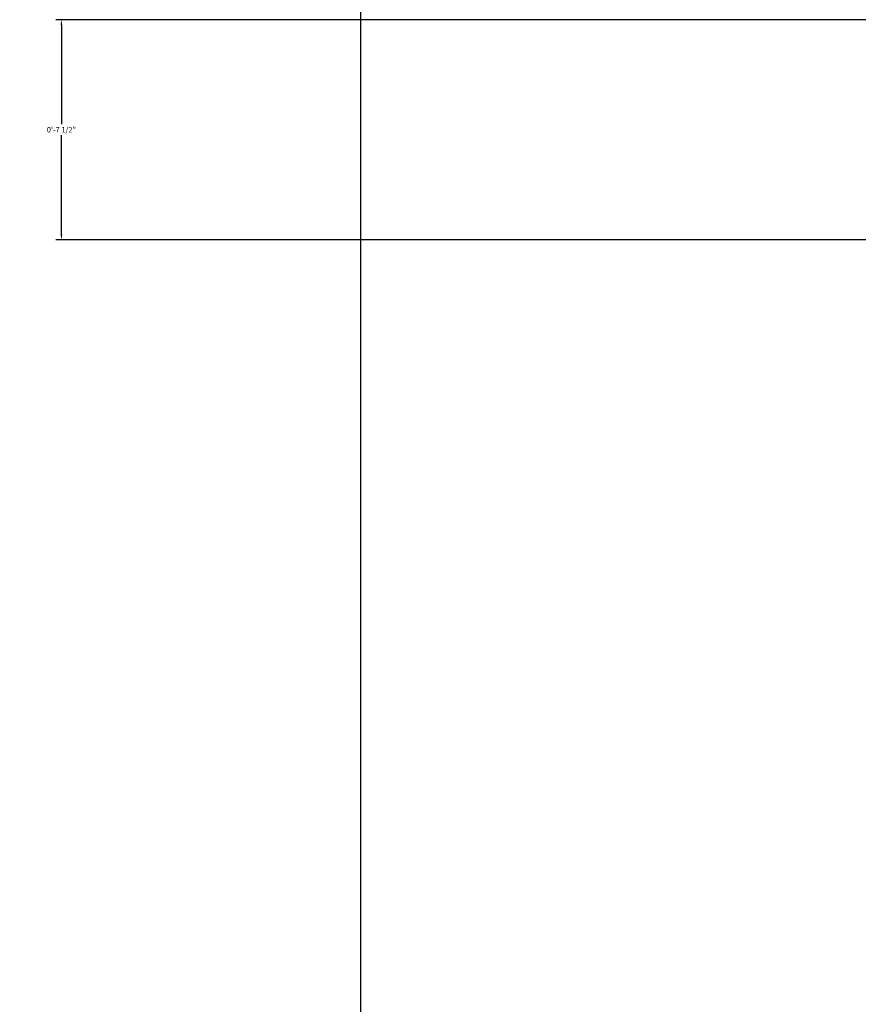
# Model space of a CAD drawing. Units: inches. Extents: x -5 to 330, y -522 to 40.
# Tile 9 of 23: x -5 to 23, y -330 to -297. Entities that reach past the tile are written whole.
import ezdxf

# ---------------------------------------------------------------- set-up
doc = ezdxf.new("R2010")
doc.units = ezdxf.units.IN
doc.header["$MEASUREMENT"] = 0
doc.layers.add('A-ANNO-DIMS', color=2, linetype='Continuous', lineweight=18)
doc.styles.get("Standard").update_dxf_attribs({"font": 'arial.ttf'})
doc.dimstyles.get("Standard").update_dxf_attribs({"dimtxt": 0.18, "dimasz": 0.18, "dimexe": 0.18, "dimexo": 0.0625, "dimgap": 0.09, "dimtad": 0, "dimtih": 1, "dimtoh": 1, "dimdec": 0, "dimzin": 0, "dimdsep": 46, "dimlunit": 3, "dimtxsty": 'Standard', "dimcen": 0.09, "dimadec": 0, "dimazin": 0, "dimtfac": 1, "dimtdec": 0, "dimtofl": 0, "dimtmove": 0, "dimatfit": 3, "dimfxl": 1, "dimtolj": 1, "dimtzin": 0, "dimarcsym": 0})

# ---------------------------------------------------------------- blocks, each defined once
blk = doc.blocks.new('*D2')
at = {"layer": 'A-ANNO-DIMS', "color": 0, "lineweight": -2, "transparency": 16777216}
for p, q in [((23.447, 12.356), (6.274, 12.356)), ((6.454, 12.176), (6.454, -203.738)), ((6.454, -425.964), (6.454, -210.049)), ((23.447, -426.144), (6.274, -426.144))]:
    blk.add_line(p, q, dxfattribs=at)
at = {"layer": 'A-ANNO-DIMS', "color": 0, "transparency": 16777216}
for points in [[(6.424, 12.176), (6.484, 12.176), (6.454, 12.356)], [(6.424, -425.964), (6.484, -425.964), (6.454, -426.144)]]:
    blk.add_solid(points, dxfattribs=at)
at = {"layer": 'Defpoints', "color": 0, "transparency": 16777216}
for p in [(23.51, 12.356), (6.454, -426.144), (23.51, -426.144)]:
    blk.add_point(p, dxfattribs=at)
at = {"layer": 'A-ANNO-DIMS', "color": 0, "transparency": 16777216, "insert": (6.454, -206.894), "char_height": 6, "attachment_point": 5}
blk.add_mtext('\\A1;36\'-7"', dxfattribs=at)
blk = doc.blocks.new('*D47')
at = {"layer": 'A-ANNO-DIMS', "color": 0, "lineweight": -2, "transparency": 16777216}
for p, q in [((32.447, -297.144), (-3.655, -297.144)), ((-3.475, -297.324), (-3.475, -300.609)), ((-3.475, -304.261), (-3.475, -300.975)), ((33.036, -304.441), (-3.655, -304.441))]:
    blk.add_line(p, q, dxfattribs=at)
at = {"layer": 'A-ANNO-DIMS', "color": 0, "transparency": 16777216}
for points in [[(-3.505, -297.324), (-3.445, -297.324), (-3.475, -297.144)], [(-3.505, -304.261), (-3.445, -304.261), (-3.475, -304.441)]]:
    blk.add_solid(points, dxfattribs=at)
at = {"layer": 'Defpoints', "color": 0, "transparency": 16777216}
for p in [(32.51, -297.144), (-3.475, -304.441), (33.099, -304.441)]:
    blk.add_point(p, dxfattribs=at)
at = {"layer": 'A-ANNO-DIMS', "color": 0, "transparency": 16777216, "insert": (-3.475, -300.792), "char_height": 0.18, "attachment_point": 5}
blk.add_mtext('\\A1;0\'-7 1/2"', dxfattribs=at)

msp = doc.modelspace()

# ---------------------------------------------------------------- dimensions: what is measured, and where the dimension line sits
at = {"layer": 'A-ANNO-DIMS'}
for base, p1, p2, override, picture, middle in [((6.454321893, -426.143582029), (23.509888577, 12.356417971), (23.509888577, -426.143582029), {"dimtxt": 6, "dimclrd": 0, "dimclre": 0, "dimclrt": 0}, '*D2', (6.454321893, -206.893582029)), ((-3.475, -304.441), (32.51, -297.144), (33.099, -304.441), {"dimdec": 1, "dimlfac": 1, "dimrnd": 0, "dimzin": 1, "dimdsep": 46, "dimlunit": 4, "dimfrac": 2}, '*D47', (-3.475, -300.792))]:
    dim = msp.add_linear_dim(base=base, p1=p1, p2=p2, angle=90, dimstyle='Standard', override=override, dxfattribs=at)
    dim.commit()
    dim.dimension.update_dxf_attribs({"geometry": picture, "text_midpoint": middle})

doc.saveas('drawing.dxf')
